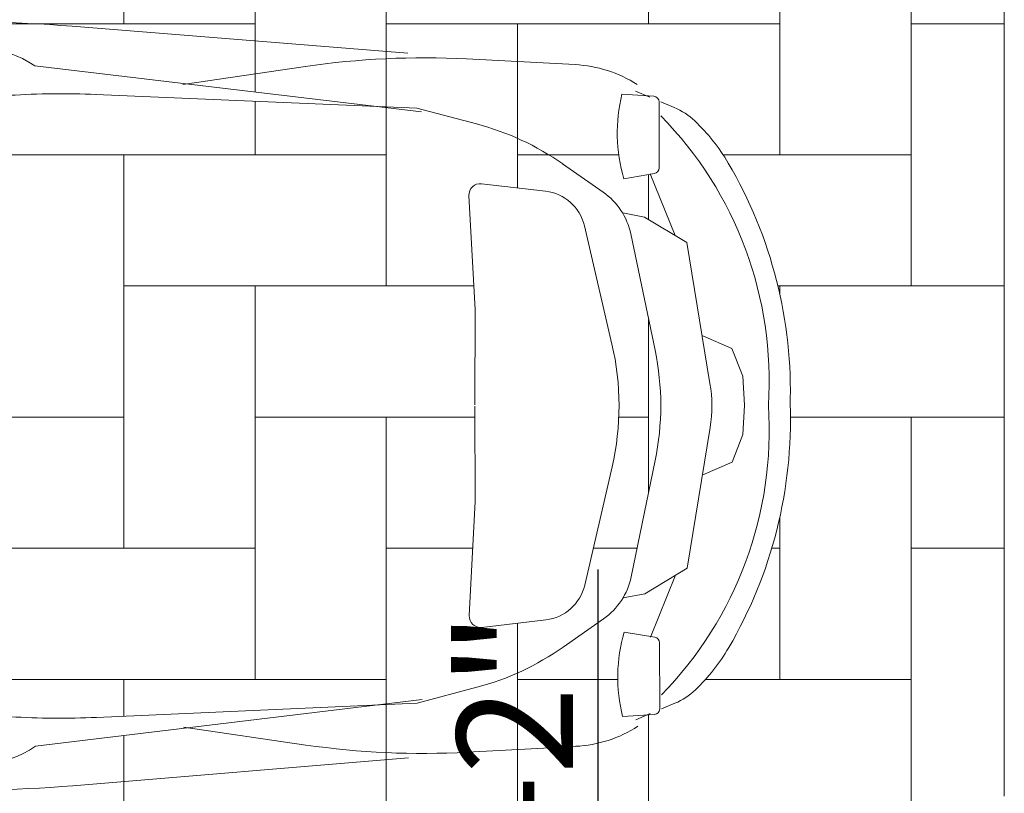
# Model space of a CAD drawing. Units: inches. Extents: x 2337 to 3570, y 1258 to 1938.
# Tile 18 of 30: x 2827 to 2903, y 1779 to 1839. Entities that reach past the tile are written whole.
import ezdxf

# ---------------------------------------------------------------- set-up
doc = ezdxf.new("R2010")
doc.units = ezdxf.units.IN
for name, color, linetype, lineweight in [('A-ANNO-DIMS', 2, 'Continuous', 18), ('A-FLOR-PATT', 252, 'Continuous', 13), ('L-SITE-GATE', 4, 'Continuous', 18), ('L-SITE-VEHI', 8, 'Continuous', 18)]:
    doc.layers.add(name, color=color, linetype=linetype, lineweight=lineweight)
doc.styles.get("Standard").update_dxf_attribs({"font": 'arial.ttf'})
doc.dimstyles.new('ISO-25', dxfattribs={"dimtxt": 9, "dimasz": 2.5, "dimexe": 1.25, "dimexo": 0.625, "dimtad": 1, "dimdec": 1, "dimlunit": 3, "dimtxsty": 'Standard', "dimcen": 2.5, "dimadec": 0, "dimazin": 0, "dimtfac": 1, "dimtdec": 1, "dimtmove": 0, "dimatfit": 3, "dimfxl": 1, "dimarcsym": 0})

# ---------------------------------------------------------------- blocks, each defined once
blk = doc.blocks.new('A$C4A3239E3')
for p, q in [((2.5445, 1.6742), (3.2816, 1.6148)), ((3.4104, 1.6024), (3.6491, 1.5899)), ((2.4629, 1.587), (3.3117, 1.4863)), ((2.7875, 1.5463), (3.0567, 1.5859)), ((2.597, 1.5244), (3.3012, 1.4943)), ((3.8218, 1.5205), (3.7519, 1.525)), ((3.7813, 1.5317), (3.8128, 1.5185)), ((3.3012, 1.4943), (3.4322, 1.4598)), ((3.8334, 1.3629), (3.8334, 1.5081)), ((3.8376, 1.5081), (3.8668, 1.4958)), ((3.6217, 1.372), (3.7108, 1.3099)), ((3.7558, 1.3393), (3.8231, 1.3506)), ((3.8137, 1.3503), (3.8686, 1.2144)), ((3.4434, 1.3284), (3.584, 1.3121)), ((3.4158, 1.3024), (3.4294, 1.0516)), ((3.7535, 1.2644), (3.8014, 1.2553)), ((3.8014, 1.2553), (3.8941, 1.199)), ((3.6693, 1.236), (3.7299, 0.9762)), ((3.7713, 1.2181), (3.8245, 0.9626)), ((3.8941, 1.199), (3.9452, 0.89)), ((3.4294, 1.0516), (3.4292, 0.8428)), ((3.9292, 0.9941), (3.9933, 0.9668)), ((3.9933, 0.9668), (4.0172, 0.906)), ((4.0172, 0.906), (4.0211, 0.842)), ((3.4299, 0.6309), (3.4292, 0.8396)), ((4.0174, 0.7775), (4.0211, 0.8416)), ((3.8948, 0.4844), (3.9453, 0.7934)), ((3.9936, 0.7167), (4.0174, 0.7775)), ((3.772, 0.465), (3.8248, 0.7206)), ((3.9295, 0.6893), (3.9936, 0.7167)), ((3.6701, 0.4469), (3.7301, 0.7068)), ((3.4167, 0.38), (3.4299, 0.6309)), ((3.8022, 0.4279), (3.8948, 0.4844)), ((3.8147, 0.3328), (3.8693, 0.4688)), ((3.7543, 0.4187), (3.8022, 0.4279)), ((3.4444, 0.354), (3.585, 0.3707)), ((3.6228, 0.3107), (3.7117, 0.3731)), ((3.7568, 0.3438), (3.8241, 0.3326)), ((3.8345, 0.3203), (3.8347, 0.1751)), ((3.3024, 0.1879), (3.4334, 0.2226)), ((2.4644, 0.0936), (3.313, 0.1959)), ((2.5984, 0.1564), (3.3024, 0.1879)), ((3.8389, 0.1752), (3.8681, 0.1875)), ((3.8231, 0.1627), (3.7532, 0.1581)), ((3.7826, 0.1514), (3.8141, 0.1647)), ((2.7889, 0.1349), (3.0581, 0.0958)), ((3.4119, 0.0799), (3.6506, 0.0929)), ((2.5461, 0.0065), (3.2831, 0.0673))]:
    blk.add_line(p, q)
for centre, radius, start, end in [((2.3053, -1.296), 2.9798, 85.3952, 92.9452), ((2.3463, 1.4226), 0.2016, 54.6492, 124.7769), ((3.3168, -0.183), 1.7879, 86.9998, 98.3676), ((3.6355, 1.3122), 0.278, 57.3299, 87.1824), ((2.5206, -0.2618), 1.7879, 87.5491, 93.6237), ((4.0973, 1.4394), 0.3558, 166.0961, 196.3535), ((3.821, 1.5081), 0.0124, 0, 86.3304), ((3.8091, 1.3584), 0.149, 46.3836, 67.2014), ((3.2466, 0.8963), 0.8285, 356.2451, 44.5195), ((3.2805, 0.8834), 0.596, 55.07, 75.2551), ((3.6181, 1.158), 0.4258, 30.4577, 46.3836), ((3.821, 1.3629), 0.0124, 279.6077, 0), ((3.1325, 0.8724), 0.9892, 358.0694, 30.4577), ((3.4406, 1.3037), 0.0248, 83.376, 183.115), ((3.5726, 1.2134), 0.0993, 13.1226, 83.376), ((3.6254, 1.1877), 0.149, 11.7694, 55.07), ((3.1495, 0.8409), 0.596, 346.9903, 13.1226), ((3.2411, 0.841), 0.596, 348.3436, 11.7694), ((3.6512, 0.8414), 0.298, 350.7246, 9.3883), ((3.1326, 0.8094), 0.9892, 329.6553, 2.0435), ((3.2467, 0.7858), 0.8285, 315.5935, 3.8679), ((3.6261, 0.4951), 0.149, 305.0429, 348.3436), ((3.5733, 0.4693), 0.0993, 276.737, 346.9903), ((3.4415, 0.3787), 0.0248, 176.9979, 276.737), ((4.0985, 0.2443), 0.3558, 163.7595, 194.0169), ((3.822, 0.3203), 0.0124, 0.113, 80.5053), ((3.2806, 0.7987), 0.596, 284.8579, 305.0429), ((3.6188, 0.5248), 0.4258, 313.7293, 329.6553), ((3.8101, 0.3247), 0.149, 292.9116, 313.7293), ((3.8223, 0.1751), 0.0124, 273.7825, 0.113), ((2.5184, 1.9425), 1.7879, 266.4893, 272.5638), ((3.6364, 0.3706), 0.278, 272.9306, 302.783), ((2.3474, 0.2577), 0.2016, 235.336, 305.4638), ((3.3148, 1.8652), 1.7879, 261.7454, 273.1132), ((2.3011, 2.9762), 2.9798, 267.1678, 274.7177)]:
    blk.add_arc(centre, radius, start, end)
blk = doc.blocks.new('*D90')
at = {"layer": 'A-ANNO-DIMS', "color": 0, "lineweight": -2, "transparency": 16777216}
for p, q in [((2871.382, 1676.497), (2871.382, 1796.695)), ((2864.515, 1676.497), (2872.632, 1676.497)), ((2871.382, 1629.048), (2871.382, 1673.997)), ((2864.515, 1626.548), (2872.632, 1626.548))]:
    blk.add_line(p, q, dxfattribs=at)
at = {"layer": 'A-ANNO-DIMS', "color": 0, "transparency": 16777216}
for points in [[(2870.966, 1673.997), (2871.799, 1673.997), (2871.382, 1676.497)], [(2870.966, 1629.048), (2871.799, 1629.048), (2871.382, 1626.548)]]:
    blk.add_solid(points, dxfattribs=at)
at = {"layer": 'Defpoints', "color": 0, "transparency": 16777216}
for p in [(2863.89, 1676.497), (2871.382, 1676.497), (2863.89, 1626.548)]:
    blk.add_point(p, dxfattribs=at)
at = {"layer": 'A-ANNO-DIMS', "color": 0, "transparency": 16777216, "insert": (2866.101, 1737.846), "char_height": 9, "attachment_point": 5, "rotation": 90}
blk.add_mtext('LOUNGE SEAT 4\'-2"', dxfattribs=at)

msp = doc.modelspace()

# ---------------------------------------------------------------- hatches: boundary and pattern name
at = {"layer": 'A-FLOR-PATT', "transparency": 33554687}
h = msp.add_hatch(dxfattribs=at)
h.set_pattern_fill('AR-HBONE', color=256, scale=0.1, angle=45)
h.paths.add_polyline_path([(2902.836, 1875.116), (2899.836, 1875.116), (2899.836, 1887.116), (2671.836, 1887.116), (2671.836, 1857.116), (2681.836, 1857.116), (2681.836, 1810.116), (2719.836, 1810.116), (2719.836, 1764.116), (2872.836, 1764.116), (2899.836, 1764.116), (2899.836, 1779.116), (2902.836, 1779.116)])
h.paths.add_polyline_path([(2854.179, 1832.557), (2857.321, 1832.422), (2861.942, 1831.206, -0.088302), (2868.629, 1828.111), (2871.77, 1825.918, -0.105467), (2873.266, 1824.315), (2874.966, 1823.992), (2877.339, 1822.551), (2875.419, 1827.303), (2873.36, 1826.955, -0.132795), (2873.22, 1833.505), (2876.098, 1833.321), (2876.098, 1832.971), (2877.275, 1832.476, -0.091085), (2878.864, 1831.436, -0.069602), (2881.45, 1828.175, -0.141553), (2886.249, 1809.409, -0.141553), (2881.487, 1790.635, -0.069602), (2878.907, 1787.369, -0.091085), (2877.321, 1786.326), (2876.14, 1785.827, -0.354729), (2875.735, 1785.451), (2873.268, 1785.288, -0.132795), (2873.395, 1791.839), (2875.455, 1791.495), (2877.365, 1796.25), (2874.995, 1794.805), (2873.296, 1794.479, -0.105467), (2871.802, 1792.873), (2868.666, 1790.673, -0.088302), (2861.985, 1787.565), (2857.366, 1786.339), (2854.225, 1786.199), (2827.803, 1783.011, -0.315912), (2819.634, 1782.954), (2793.542, 1785.741), (2798.79, 1786.943), (2825.847, 1785.283, 0.026512), (2832.53, 1785.227), (2857.366, 1786.339), (2861.985, 1787.565, 0.088302), (2868.666, 1790.673), (2871.802, 1792.873, 0.191215), (2873.932, 1796.114), (2875.792, 1805.131, 0.102572), (2875.784, 1813.667), (2873.906, 1822.681, 0.191215), (2871.77, 1825.918), (2868.629, 1828.111, 0.088302), (2861.942, 1831.206), (2857.321, 1832.422), (2832.483, 1833.486, 0.026512), (2825.799, 1833.417), (2798.745, 1831.704), (2793.496, 1832.895), (2819.582, 1835.733, -0.315912), (2827.751, 1835.692)], flags=16)
h.paths.add_polyline_path([(2862.34, 1826.572), (2867.3, 1825.996, -0.316515), (2870.308, 1823.311), (2872.444, 1814.149, -0.11452), (2872.453, 1804.643), (2870.336, 1795.477, -0.316515), (2867.333, 1792.786), (2862.374, 1792.2, -0.464922), (2861.397, 1793.116), (2861.861, 1801.965), (2861.836, 1809.385), (2861.846, 1816.806), (2861.365, 1825.654, -0.464922)], flags=16)
h.paths.add_polyline_path([(2821.293, 1791.09), (2807.573, 1791.499, -0.405226), (2805.023, 1794.123), (2805.023, 1794.121, 0.40508), (2807.573, 1791.499), (2821.293, 1791.09, 0.423258), (2823.999, 1793.719), (2823.999, 1793.719, -0.423258)], flags=16)
h.paths.add_polyline_path([(2879.429, 1814.798), (2881.737, 1813.816), (2882.582, 1811.673), (2882.717, 1809.406), (2882.586, 1807.139), (2881.746, 1804.994), (2879.439, 1804.008), (2880.042, 1807.699, 0.081616), (2880.039, 1811.108)], flags=0)
h.paths.add_polyline_path([(2796.957, 1829.715), (2796.14, 1815.428, 0.029076), (2796.152, 1803.213), (2796.997, 1788.928, -0.409057), (2796.19, 1788.002), (2791.055, 1787.607), (2785.763, 1792.935, -0.173254), (2784.26, 1796.136), (2783.472, 1804.33, -0.047466), (2783.462, 1814.286), (2784.234, 1822.482, -0.173254), (2785.73, 1825.686), (2791.012, 1831.024), (2796.148, 1830.639, -0.409057)], flags=16)
h.paths.add_polyline_path([(2750.344, 1835.795), (2750.012, 1834.37, 0.040009), (2748.771, 1826.064), (2748.631, 1824.022), (2750.526, 1825.239), (2756.614, 1827.237), (2771.951, 1829.419), (2781.401, 1831.049), (2780.099, 1822.888), (2779.438, 1814.328), (2779.144, 1809.304), (2779.447, 1804.281), (2780.126, 1795.721), (2781.444, 1787.563), (2771.99, 1789.174), (2756.65, 1791.337), (2750.557, 1793.323), (2748.66, 1794.536), (2748.804, 1792.494, 0.040009), (2750.062, 1784.191), (2750.396, 1782.767), (2745.899, 1784.642), (2744.102, 1788.129), (2743.099, 1791.925), (2741.068, 1802.995), (2740.859, 1809.271), (2741.055, 1815.548), (2743.065, 1826.622), (2744.061, 1830.421), (2745.851, 1833.911)], flags=16)
h.paths.add_polyline_path([(2761.183, 1831.202), (2754.851, 1829.51), (2754.556, 1830.832, -0.143032), (2754.62, 1831.812), (2755.053, 1833), (2761.169, 1831.713, -0.789416)], flags=16)
h.paths.add_polyline_path([(2761.226, 1787.381), (2754.89, 1789.061), (2754.599, 1787.738, 0.143032), (2754.665, 1786.758), (2755.1, 1785.571), (2761.213, 1786.87, 0.789416)], flags=16)
h.paths.add_polyline_path([(2689.028, 1816.171), (2701.274, 1816.171), (2701.274, 1823.798), (2689.028, 1823.798)], flags=24)
h.paths.add_polyline_path([(2755.384, 1858.953), (2808.715, 1858.953), (2808.715, 1885.073), (2755.384, 1885.073)], flags=24)

# ---------------------------------------------------------------- linework, layer by layer
at = {"layer": 'L-SITE-GATE'}
msp.add_line((2902.836, 1875.116), (2902.836, 1779.116), dxfattribs=at)

# ---------------------------------------------------------------- block references
at = {"layer": 'L-SITE-VEHI', "xscale": 35.27598425228, "yscale": 35.27598425228, "zscale": 35.27598425228}
msp.add_blockref('A$C4A3239E3', (2740.869, 1779.711), dxfattribs=at)

# ---------------------------------------------------------------- dimensions: what is measured, and where the dimension line sits
at = {"layer": 'A-ANNO-DIMS'}
dim = msp.add_linear_dim(base=(2871.382, 1676.497), p1=(2863.89, 1626.548), p2=(2863.89, 1676.497), angle=90, text='LOUNGE SEAT <>', dimstyle='ISO-25', override={"dimdec": 1, "dimlfac": 1, "dimrnd": 0, "dimzin": 1, "dimdsep": 46, "dimlunit": 4, "dimfrac": 2}, dxfattribs=at)
dim.commit()
dim.dimension.update_dxf_attribs({"geometry": '*D90', "text_midpoint": (2866.101, 1737.846)})

doc.saveas('drawing.dxf')
